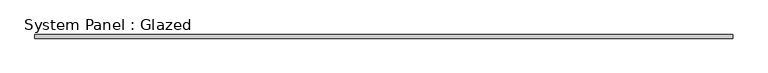
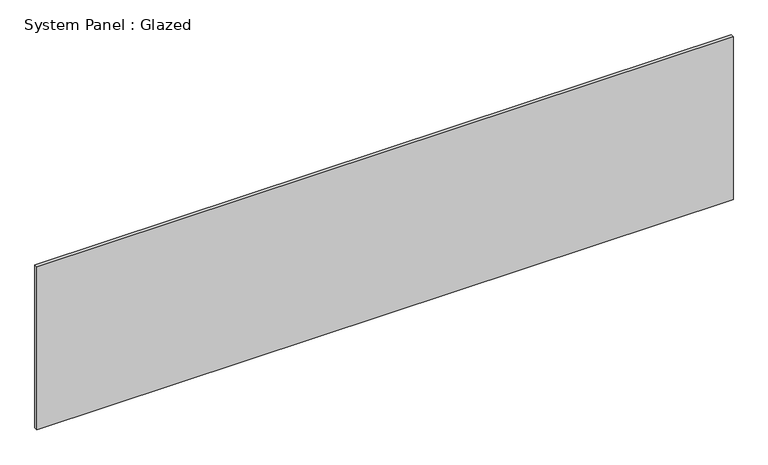
"""IFC4 building model written with IfcOpenShell, lengths in millimetres: plate geometry, System Panel : Glazed."""

from ifc_helpers import new_model, si_unit, origin, origin_with_axes, place, context, project, spatial, polyline, outline, extrude, source, transform, mapped, element, save


def system_panel_glazed_21912a48(model_context):
    return source(origin(), model_context, "Body", "SweptSolid", [
        extrude(outline(polyline([(2462.4718784, 19.05), (-2462.4718784, 19.05), (-2462.4718784, 44.45), (2462.4718784, 44.45), (2462.4718784, 19.05)])), origin_with_axes(), (0.0, 0.0, 1.0), 1219.2),
    ])


if __name__ == "__main__":
    model = new_model("IFC4")
    model_context = context("Model", 3, world=origin())
    ifc_project = project(units=[si_unit("LENGTHUNIT", "METRE", prefix="MILLI")], contexts=[model_context])
    site = spatial("IfcSite", under=ifc_project)
    building = spatial("IfcBuilding", under=site)
    placement = place(None, origin())
    system_panel_glazed_shape = system_panel_glazed_21912a48(model_context)
    element("IfcPlate", 1, ObjectType="System Panel : Glazed", at=placement, inside=building, context=model_context, shape_type="MappedRepresentation", body=[
        mapped(system_panel_glazed_shape, transform((0.0, 0.0, 0.0), x_axis=(1.0, 0.0, 0.0), y_axis=(0.0, 1.0, 0.0), z_axis=(0.0, 0.0, 1.0))),
    ])
    save(model, "model.ifc")

# Revit data of these elements
# Type "System Panel : Glazed"
#   Construction Type Id = "GSP4R"
#   Analytic Construction = "1/8 in Pilkington single glazing"
#   Visual Light Transmittance = 0.9
#   Solar Heat Gain Coefficient = 0.86
#   Heat Transfer Coefficient (U) = 1.18115 BTU/(h·ft²·°F)
# Element 1 (IfcPlate, "System Panel : Glazed")
#   Materials on its faces: "Glass"
# Materials
#   "Glass": class "Glass", colour RGB 0 128 192, transparency 0.75, Description = "Soda Lime Glass", Cost = 0
